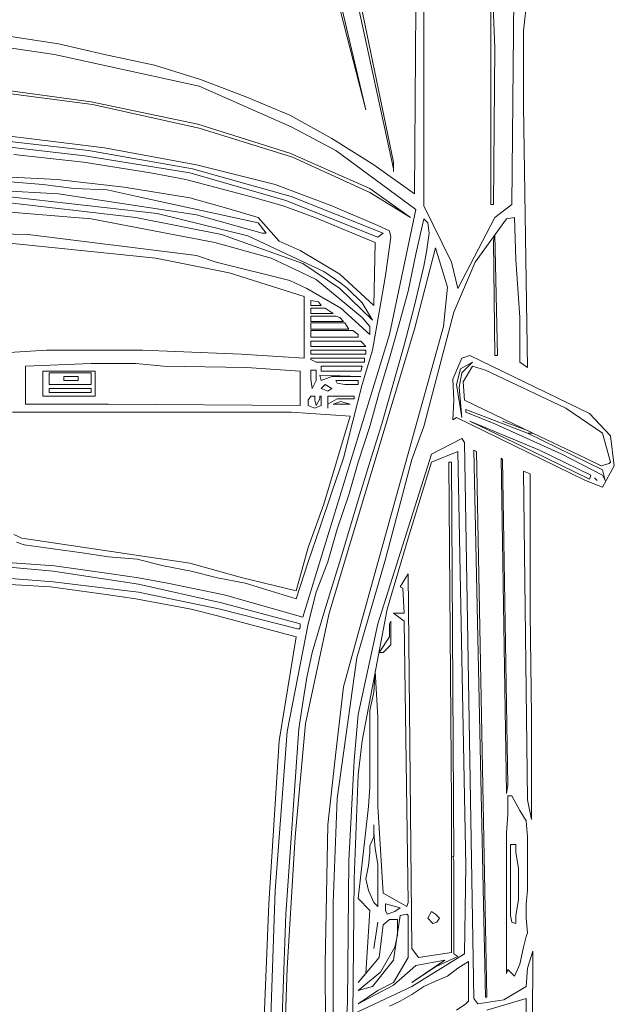
# Model space of a CAD drawing. Units: inches. Extents: x -9 to 646, y -802 to 47.
# Tile 8 of 17: x 465 to 490, y -602 to -561. Entities that reach past the tile are written whole.
import ezdxf

# ---------------------------------------------------------------- set-up
doc = ezdxf.new("R2010")
doc.units = ezdxf.units.IN
doc.header["$MEASUREMENT"] = 0
doc.layers.add('A-SITE-VEHI', color=8, linetype='Continuous', lineweight=9)

msp = doc.modelspace()

# ---------------------------------------------------------------- linework, layer by layer
at = {"layer": 'A-SITE-VEHI'}
for p, q in [((474.722, -545.354), (479.383, -565.082)), ((484.206, -549.797), (484.694, -562.536)), ((480.522, -567.521), (476.836, -550.556)), ((481.767, -550.827), (481.767, -569.039)), ((477.54, -552.941), (480.522, -567.25)), ((485.398, -568.984), (485.507, -558.523)), ((479.383, -565.082), (477.811, -558.958)), ((485.886, -561.83), (486.048, -560.313)), ((481.388, -568.551), (481.443, -560.855)), ((484.532, -568.984), (484.532, -560.964)), ((485.886, -564.92), (485.886, -561.83)), ((466.537, -562.806), (462.418, -562.209)), ((464.639, -562.047), (466.699, -562.371)), ((466.699, -562.371), (468.596, -562.806)), ((484.694, -562.536), (484.641, -568.984)), ((472.499, -564.108), (466.537, -562.806)), ((468.596, -562.806), (470.656, -563.239)), ((470.656, -563.239), (472.553, -563.835)), ((472.553, -563.835), (474.396, -564.541)), ((463.069, -564.214), (468.109, -564.865)), ((468.054, -564.756), (463.231, -564.108)), ((476.294, -565.786), (472.499, -564.108)), ((474.396, -564.541), (476.239, -565.3)), ((472.444, -565.678), (468.054, -564.756)), ((468.109, -564.865), (472.499, -565.842)), ((486.048, -575.705), (485.886, -564.92)), ((476.239, -565.3), (477.973, -566.275)), ((476.239, -566.87), (472.444, -565.678)), ((472.499, -565.842), (476.347, -567.034)), ((478.137, -566.763), (476.294, -565.786)), ((467.945, -566.763), (463.611, -566.275)), ((468.596, -566.655), (464.694, -566.166)), ((477.973, -566.275), (479.707, -567.358)), ((463.502, -566.492), (467.783, -566.979)), ((472.39, -567.358), (468.596, -566.655)), ((467.73, -567.25), (464.856, -566.925)), ((467.783, -566.979), (472.12, -567.685)), ((472.228, -567.521), (467.945, -566.763)), ((479.545, -568.335), (476.239, -566.87)), ((476.347, -567.034), (479.545, -568.497)), ((481.443, -569.201), (478.137, -566.763)), ((458.026, -567.521), (466.646, -567.956)), ((470.494, -567.685), (467.73, -567.25)), ((476.294, -568.66), (472.228, -567.521)), ((475.643, -568.171), (472.39, -567.358)), ((479.707, -567.358), (481.388, -568.551)), ((480.522, -567.25), (480.522, -567.629)), ((471.957, -567.956), (470.494, -567.685)), ((472.12, -567.685), (476.076, -568.822)), ((458.948, -568.118), (466.699, -568.551)), ((466.049, -568.171), (463.447, -567.956)), ((467.35, -568.335), (466.049, -568.171)), ((466.646, -567.956), (469.411, -568.28)), ((468.705, -568.389), (467.35, -568.335)), ((469.411, -568.28), (472.12, -568.713)), ((474.613, -568.66), (471.957, -567.956)), ((477.973, -569.039), (475.643, -568.171)), ((481.226, -569.528), (479.545, -568.335)), ((470.765, -569.364), (463.664, -568.551)), ((466.699, -568.551), (472.39, -569.419)), ((469.952, -568.66), (468.705, -568.389)), ((474.937, -569.743), (469.952, -568.66)), ((472.12, -568.713), (473.692, -569.148)), ((475.968, -569.039), (474.613, -568.66)), ((480.087, -570.176), (476.294, -568.66)), ((479.545, -568.497), (481.226, -569.528)), ((463.826, -568.822), (469.897, -569.528)), ((477.269, -569.528), (475.968, -569.039)), ((476.076, -568.822), (479.871, -570.34)), ((479.871, -569.852), (477.973, -569.039)), ((481.767, -569.039), (482.906, -571.369)), ((484.641, -568.984), (484.532, -568.984)), ((484.694, -569.528), (485.398, -568.984)), ((468.054, -569.581), (462.798, -569.148)), ((469.897, -569.528), (473.421, -570.232)), ((474.504, -570.285), (470.765, -569.364)), ((472.39, -569.419), (475.102, -570.176)), ((473.692, -569.148), (474.937, -569.528)), ((474.937, -569.528), (475.806, -570.503)), ((479.762, -570.556), (477.269, -569.528)), ((480.357, -574.351), (481.443, -569.201)), ((483.177, -572.454), (484.694, -569.528)), ((485.182, -569.581), (485.507, -569.528)), ((485.507, -569.528), (485.562, -571.262)), ((473.15, -570.556), (468.054, -569.581)), ((475.264, -570.176), (474.937, -569.743)), ((480.357, -570.07), (479.871, -569.852)), ((481.767, -569.581), (481.443, -571.044)), ((481.93, -569.743), (481.767, -569.581)), ((481.985, -570.176), (481.93, -569.743)), ((483.881, -571.369), (485.182, -569.581)), ((463.069, -570.176), (465.454, -570.232)), ((465.454, -570.232), (472.39, -571.098)), ((473.421, -570.232), (476.78, -571.424)), ((477.648, -571.748), (474.504, -570.285)), ((475.102, -570.176), (475.264, -570.176)), ((479.871, -570.34), (480.087, -570.176)), ((480.195, -571.913), (480.413, -570.34)), ((480.413, -570.34), (480.357, -570.07)), ((481.876, -570.936), (481.985, -570.176)), ((484.694, -570.232), (484.641, -570.503)), ((484.803, -575.219), (484.694, -570.232)), ((470.71, -571.206), (464.423, -570.556)), ((475.479, -571.206), (473.15, -570.556)), ((475.806, -570.503), (476.672, -570.882)), ((479.707, -573.158), (479.762, -570.556)), ((484.641, -570.503), (484.694, -575.219)), ((472.39, -571.098), (473.203, -571.369)), ((476.672, -570.882), (478.299, -571.857)), ((481.443, -571.044), (481.117, -572.561)), ((481.388, -574.133), (482.256, -570.773)), ((481.767, -571.533), (481.876, -570.936)), ((482.256, -570.773), (482.742, -572.399)), ((473.745, -571.804), (470.71, -571.206)), ((473.203, -571.369), (476.239, -572.128)), ((476.401, -571.642), (475.479, -571.206)), ((476.78, -571.424), (478.299, -572.454)), ((481.388, -573.158), (481.767, -571.533)), ((482.906, -571.369), (483.177, -572.454)), ((483.013, -573.429), (483.881, -571.369)), ((485.562, -571.262), (485.724, -573.647)), ((476.836, -572.779), (473.745, -571.804)), ((477.322, -572.075), (476.401, -571.642)), ((478.352, -572.237), (477.648, -571.748)), ((478.299, -571.857), (479.707, -573.158)), ((479.924, -573.429), (480.195, -571.913)), ((476.239, -572.128), (476.945, -572.454)), ((479.221, -573.647), (477.322, -572.075)), ((478.623, -572.454), (478.352, -572.237)), ((476.836, -575.325), (476.836, -572.779)), ((476.945, -572.454), (478.352, -573.267)), ((478.299, -572.454), (479.654, -573.755)), ((479.221, -573.049), (478.623, -572.454)), ((481.117, -572.561), (480.737, -573.971)), ((482.742, -572.399), (482.58, -574.026)), ((477.431, -572.996), (477.107, -572.941)), ((477.107, -572.941), (477.107, -573.158)), ((477.107, -573.158), (477.54, -573.158)), ((477.54, -573.158), (477.431, -572.996)), ((479.654, -573.755), (479.221, -573.049)), ((480.955, -574.784), (481.388, -573.158)), ((477.702, -573.267), (477.107, -573.267)), ((477.107, -573.267), (477.107, -573.482)), ((477.107, -573.482), (478.028, -573.482)), ((478.137, -573.591), (477.107, -573.591)), ((477.107, -573.591), (477.107, -573.809)), ((478.028, -573.482), (477.702, -573.267)), ((478.299, -573.647), (478.137, -573.591)), ((478.352, -573.267), (479.545, -574.351)), ((479.654, -575.001), (479.924, -573.429)), ((481.767, -578.145), (483.013, -573.429)), ((477.107, -573.809), (478.461, -573.809)), ((478.514, -573.862), (477.107, -573.862)), ((477.107, -573.862), (477.107, -574.133)), ((478.461, -573.809), (478.299, -573.647)), ((478.679, -574.133), (478.514, -573.862)), ((479.545, -574.026), (479.221, -573.647)), ((480.737, -573.971), (480.357, -575.325)), ((485.724, -573.647), (485.724, -575.49)), ((476.78, -586.004), (480.357, -574.351)), ((477.107, -574.133), (478.679, -574.133)), ((478.841, -574.189), (477.107, -574.189)), ((477.107, -574.189), (477.107, -574.459)), ((477.864, -585.841), (481.388, -574.133)), ((479.058, -574.351), (478.841, -574.189)), ((479.058, -574.459), (479.058, -574.351)), ((482.58, -574.026), (479.165, -586.274)), ((479.545, -574.351), (479.545, -574.026)), ((477.107, -574.459), (479.058, -574.459)), ((479.165, -574.622), (477.107, -574.622)), ((477.107, -574.622), (477.107, -574.839)), ((479.221, -574.675), (479.165, -574.622)), ((479.383, -574.839), (479.221, -574.675)), ((480.033, -578.037), (480.955, -574.784)), ((463.502, -575.163), (466.211, -575.001)), ((466.211, -575.001), (470.168, -575.001)), ((470.168, -575.001), (471.524, -575.055)), ((471.524, -575.055), (474.233, -575.163)), ((474.233, -575.163), (476.836, -575.325)), ((477.107, -574.839), (479.383, -574.839)), ((479.383, -575.001), (477.107, -575.001)), ((477.107, -575.001), (477.107, -575.163)), ((477.107, -575.163), (479.383, -575.163)), ((479.221, -576.411), (479.654, -575.001)), ((479.383, -575.163), (479.383, -575.001)), ((483.664, -575.219), (483.339, -575.325)), ((488.597, -577.604), (483.664, -575.219)), ((484.694, -575.219), (484.803, -575.219)), ((468.054, -575.543), (465.345, -575.652)), ((469.897, -575.543), (468.054, -575.543)), ((471.036, -575.652), (469.897, -575.543)), ((479.329, -575.325), (477.107, -575.325)), ((477.107, -575.325), (477.107, -575.381)), ((477.107, -575.381), (477.322, -575.49)), ((477.322, -575.49), (479.329, -575.49)), ((479.329, -575.49), (479.329, -575.325)), ((480.357, -575.325), (479.924, -576.735)), ((483.339, -575.325), (482.96, -576.194)), ((483.772, -575.49), (483.284, -575.761)), ((483.339, -575.923), (483.772, -575.49)), ((485.724, -575.49), (486.048, -575.705)), ((465.345, -575.652), (465.345, -577.224)), ((468.218, -575.867), (466.049, -575.867)), ((466.049, -575.867), (466.049, -576.897)), ((468.054, -575.923), (466.32, -575.923)), ((466.32, -575.923), (466.32, -576.411)), ((468.054, -576.411), (468.054, -575.923)), ((468.218, -576.897), (468.218, -575.867)), ((474.451, -575.705), (471.036, -575.652)), ((476.672, -575.867), (474.451, -575.705)), ((476.672, -577.277), (476.672, -575.867)), ((477.322, -575.814), (477.107, -575.814)), ((477.107, -575.814), (477.107, -576.194)), ((477.322, -576.247), (477.322, -575.814)), ((479.165, -576.085), (477.486, -576.031)), ((477.486, -576.031), (477.54, -576.247)), ((479.221, -575.652), (477.54, -575.652)), ((477.54, -575.652), (477.54, -575.867)), ((477.54, -575.867), (479.165, -575.867)), ((479.165, -575.867), (479.221, -575.652)), ((483.284, -575.761), (483.122, -576.411)), ((483.231, -576.518), (483.339, -575.923)), ((483.772, -575.652), (483.393, -576.302)), ((484.314, -575.814), (483.772, -575.652)), ((487.621, -577.386), (484.314, -575.814)), ((466.32, -576.411), (468.054, -576.411)), ((467.512, -576.085), (466.917, -576.085)), ((466.917, -576.085), (466.917, -576.247)), ((466.917, -576.247), (467.512, -576.247)), ((467.512, -576.247), (467.512, -576.085)), ((477.107, -576.194), (477.16, -576.573)), ((477.16, -576.573), (477.322, -576.247)), ((477.54, -576.247), (477.973, -576.085)), ((477.702, -576.411), (477.54, -576.573)), ((477.973, -576.573), (477.702, -576.411)), ((477.973, -576.085), (479.165, -576.085)), ((479.058, -576.247), (478.137, -576.247)), ((478.137, -576.247), (478.19, -576.356)), ((478.19, -576.356), (478.514, -576.411)), ((478.514, -576.411), (479.058, -576.411)), ((478.841, -577.928), (479.221, -576.411)), ((479.058, -576.411), (479.058, -576.247)), ((482.96, -576.194), (483.013, -577.062)), ((483.122, -576.411), (483.339, -577.766)), ((483.393, -576.302), (483.448, -577.062)), ((468.054, -576.573), (466.32, -576.573)), ((466.32, -576.573), (466.32, -576.735)), ((466.32, -576.735), (468.054, -576.735)), ((468.054, -576.735), (468.054, -576.573)), ((477.54, -576.573), (477.811, -576.682)), ((477.811, -576.682), (477.973, -576.573)), ((479.924, -576.735), (479.545, -578.145)), ((483.339, -577.766), (483.231, -576.518)), ((465.345, -577.224), (468.76, -577.224)), ((466.049, -576.897), (468.218, -576.897)), ((468.76, -577.224), (476.672, -577.277)), ((477.107, -576.897), (476.998, -577.062)), ((476.998, -577.062), (476.998, -577.277)), ((477.269, -576.897), (477.107, -576.897)), ((477.269, -577.062), (477.269, -576.897)), ((477.322, -577.277), (477.269, -577.062)), ((477.486, -577.006), (477.322, -577.277)), ((477.54, -576.897), (477.486, -576.897)), ((477.486, -576.897), (477.486, -577.006)), ((477.54, -577.277), (477.54, -576.897)), ((478.894, -576.897), (477.811, -576.897)), ((477.811, -576.897), (477.811, -577.386)), ((477.811, -577.224), (478.19, -577.006)), ((478.352, -577.115), (478.028, -577.224)), ((478.028, -577.224), (478.732, -577.224)), ((478.19, -577.006), (478.894, -577.006)), ((478.732, -577.224), (478.352, -577.115)), ((478.894, -577.006), (478.894, -576.897)), ((483.013, -577.062), (482.96, -577.874)), ((483.448, -577.062), (486.266, -578.416)), ((476.294, -577.548), (464.803, -577.548)), ((478.732, -577.71), (476.294, -577.548)), ((476.998, -577.277), (477.269, -577.386)), ((477.269, -577.386), (477.54, -577.277)), ((486.048, -578.416), (483.502, -577.439)), ((483.502, -577.439), (483.502, -577.548)), ((483.502, -577.548), (484.694, -578.037)), ((489.139, -578.416), (487.621, -577.386)), ((489.464, -578.525), (488.597, -577.604)), ((477.648, -581.343), (478.732, -577.71)), ((478.461, -579.447), (478.841, -577.928)), ((479.545, -579.609), (480.033, -578.037)), ((482.96, -577.874), (483.122, -577.766)), ((483.122, -577.766), (488.433, -580.368)), ((483.664, -577.928), (486.266, -579.176)), ((486.537, -579.12), (483.664, -577.928)), ((484.694, -578.037), (487.458, -579.282)), ((485.02, -577.928), (486.048, -578.307)), ((479.545, -578.145), (479.058, -579.609)), ((481.279, -579.5), (481.767, -578.145)), ((489.139, -579.933), (486.048, -578.416)), ((486.048, -578.416), (486.266, -578.416)), ((486.266, -578.416), (488.433, -579.447)), ((489.464, -579.609), (489.139, -578.416)), ((483.339, -578.632), (482.092, -579.282)), ((483.448, -578.796), (483.339, -578.632)), ((483.828, -601.722), (483.448, -578.796)), ((489.626, -579.771), (489.464, -578.525)), ((482.092, -579.282), (479.871, -586.274)), ((483.177, -579.176), (482.092, -579.609)), ((483.502, -596.249), (483.177, -579.176)), ((483.935, -579.176), (483.828, -579.12)), ((483.828, -579.12), (484.314, -601.669)), ((484.37, -601.669), (483.935, -579.176)), ((486.266, -579.176), (488.597, -580.313)), ((488.651, -580.15), (486.537, -579.12)), ((487.458, -579.282), (489.139, -580.15)), ((477.973, -580.854), (478.461, -579.447)), ((479.058, -579.609), (478.679, -580.963)), ((479.058, -581.181), (479.545, -579.609)), ((480.195, -583.619), (481.279, -579.5)), ((482.092, -579.609), (481.117, -582.753)), ((482.906, -579.609), (482.798, -579.609)), ((482.798, -579.609), (482.906, -593.7)), ((483.013, -595.869), (482.906, -579.609)), ((485.02, -579.5), (484.965, -579.447)), ((484.965, -579.447), (485.182, -593.267)), ((485.236, -592.942), (485.02, -579.5)), ((488.433, -579.447), (489.084, -579.771)), ((489.084, -579.771), (489.41, -579.662)), ((489.41, -579.662), (489.464, -579.609)), ((486.157, -580.095), (485.886, -579.988)), ((485.886, -579.988), (486.048, -593.538)), ((486.157, -585.841), (486.157, -580.095)), ((489.139, -580.639), (489.626, -579.771)), ((489.248, -580.368), (489.139, -579.933)), ((488.433, -580.368), (489.139, -580.639)), ((488.597, -580.313), (488.651, -580.15)), ((488.813, -580.259), (488.922, -580.368)), ((489.139, -580.15), (489.248, -580.368)), ((477.486, -582.318), (477.973, -580.854)), ((478.679, -580.963), (478.19, -582.373)), ((478.352, -583.565), (479.058, -581.181)), ((476.998, -583.13), (477.648, -581.343)), ((476.998, -583.728), (477.486, -582.318)), ((478.19, -582.373), (477.811, -583.728)), ((464.856, -582.589), (465.183, -582.753)), ((464.965, -582.915), (465.29, -583.024)), ((465.183, -582.753), (472.12, -583.781)), ((481.117, -582.753), (480.251, -585.679)), ((465.29, -583.024), (467.674, -583.348)), ((467.674, -583.348), (468.76, -583.51)), ((476.509, -584.92), (476.998, -583.13)), ((462.905, -583.619), (466.537, -583.89)), ((468.76, -583.51), (469.952, -583.619)), ((469.952, -583.619), (471.036, -583.89)), ((476.509, -585.244), (476.998, -583.728)), ((477.811, -583.728), (477.322, -584.973)), ((477.648, -585.841), (478.352, -583.565)), ((479.003, -587.684), (480.195, -583.619)), ((466.482, -584.107), (462.905, -583.781)), ((470.006, -584.649), (466.482, -584.107)), ((466.537, -583.89), (468.867, -584.216)), ((471.036, -583.89), (472.173, -584.107)), ((472.12, -583.781), (474.287, -584.378)), ((472.173, -584.107), (473.259, -584.378)), ((466.375, -584.758), (462.798, -584.54)), ((462.905, -584.269), (466.482, -584.54)), ((466.482, -584.54), (470.006, -584.973)), ((468.867, -584.216), (470.006, -584.378)), ((470.006, -584.378), (471.198, -584.596)), ((473.259, -584.378), (474.396, -584.596)), ((474.287, -584.378), (476.509, -584.92)), ((481.117, -584.216), (480.793, -584.758)), ((481.279, -599.662), (481.117, -584.216)), ((468.76, -585.082), (466.375, -584.758)), ((473.421, -585.408), (470.006, -584.649)), ((470.006, -584.973), (473.365, -585.679)), ((471.198, -584.596), (473.53, -585.082)), ((474.396, -584.596), (475.426, -584.92)), ((475.426, -584.92), (476.509, -585.244)), ((477.322, -584.973), (476.998, -586.274)), ((480.793, -584.758), (480.899, -584.811)), ((480.899, -584.811), (480.955, -585.841)), ((469.897, -585.244), (468.76, -585.082)), ((472.173, -585.679), (469.897, -585.244)), ((473.53, -585.082), (476.78, -586.004)), ((473.259, -585.95), (472.173, -585.679)), ((473.365, -585.679), (476.618, -586.492)), ((476.672, -586.274), (473.421, -585.408)), ((480.251, -585.679), (479.221, -591.099)), ((476.509, -586.816), (473.259, -585.95)), ((476.889, -590.393), (477.864, -585.841)), ((477.16, -587.467), (477.648, -585.841)), ((480.413, -586.166), (480.357, -586.274)), ((480.413, -587.143), (480.413, -586.166)), ((480.955, -585.841), (480.522, -585.841)), ((480.522, -585.841), (480.955, -586.166)), ((480.955, -586.166), (481.117, -597.765)), ((486.213, -590.069), (486.157, -585.841)), ((476.998, -586.274), (476.13, -590.72)), ((476.618, -586.492), (476.672, -586.437)), ((476.672, -586.437), (476.672, -586.274)), ((479.165, -586.274), (478.461, -588.877)), ((479.871, -586.274), (479.058, -590.016)), ((480.357, -586.274), (480.357, -586.816)), ((475.806, -591.099), (476.509, -586.816)), ((480.357, -586.816), (479.924, -587.467)), ((480.087, -587.467), (480.413, -587.143)), ((476.945, -588.497), (477.16, -587.467)), ((478.19, -593.484), (479.003, -587.684)), ((479.924, -587.467), (480.087, -587.467)), ((479.762, -588.226), (479.707, -589.094)), ((479.871, -590.122), (479.762, -588.226)), ((476.78, -589.527), (476.945, -588.497)), ((478.461, -588.877), (478.137, -591.586)), ((479.707, -589.094), (479.545, -589.852)), ((476.618, -590.611), (476.78, -589.527)), ((479.058, -590.016), (478.894, -591.912)), ((479.545, -589.852), (479.545, -592.996)), ((479.871, -593.808), (479.871, -590.122)), ((486.213, -594.35), (486.213, -590.069)), ((476.076, -598.254), (476.618, -590.611)), ((476.456, -595.056), (476.889, -590.393)), ((476.13, -590.72), (475.643, -597.277)), ((475.372, -597.821), (475.806, -591.099)), ((479.221, -591.099), (479.058, -592.507)), ((478.137, -591.586), (477.811, -594.568)), ((478.894, -591.912), (478.679, -596.031)), ((479.058, -592.507), (478.894, -596.79)), ((479.545, -592.996), (479.491, -593.808)), ((485.182, -593.267), (485.236, -592.942)), ((478.028, -597.765), (478.19, -593.484)), ((485.398, -593.375), (485.236, -593.375)), ((485.236, -593.375), (485.236, -594.135)), ((485.724, -593.971), (485.398, -593.375)), ((479.491, -593.808), (479.058, -597.603)), ((480.087, -597.386), (479.871, -593.808)), ((482.906, -593.7), (482.906, -599.826)), ((486.048, -593.538), (486.213, -594.35)), ((485.236, -594.135), (485.182, -594.892)), ((485.995, -594.406), (485.724, -593.971)), ((477.811, -594.568), (477.702, -600.312)), ((479.707, -594.568), (479.707, -595.056)), ((486.048, -595.056), (485.995, -594.406)), ((476.13, -600.476), (476.456, -595.056)), ((479.707, -595.056), (479.545, -595.436)), ((479.762, -595.543), (479.707, -594.892)), ((485.182, -594.892), (485.182, -600.692)), ((486.048, -597.277), (486.048, -595.056)), ((479.545, -595.436), (479.545, -595.707)), ((485.562, -595.38), (485.345, -595.38)), ((485.345, -595.38), (485.345, -598.307)), ((485.562, -595.707), (485.562, -595.38)), ((479.545, -595.707), (479.491, -596.249)), ((479.871, -596.193), (479.762, -595.543)), ((483.013, -596.031), (482.96, -595.869)), ((482.96, -595.869), (483.013, -595.869)), ((485.671, -596.355), (485.562, -595.707)), ((478.679, -596.031), (478.623, -601.884)), ((479.491, -596.249), (479.383, -596.79)), ((479.871, -597.927), (479.871, -596.193)), ((483.013, -599.879), (483.013, -596.031)), ((483.448, -599.879), (483.502, -596.249)), ((485.671, -597.656), (485.671, -596.355)), ((478.894, -596.79), (478.841, -602.373)), ((479.383, -596.79), (479.491, -597.277)), ((475.643, -597.277), (474.451, -630.612)), ((479.491, -597.277), (479.707, -597.765)), ((481.064, -597.927), (480.087, -597.386)), ((485.995, -597.821), (486.048, -597.277)), ((475.102, -604.487), (475.372, -597.821)), ((478.028, -603.727), (478.028, -597.765)), ((479.058, -597.603), (479.545, -598.092)), ((479.707, -597.765), (479.871, -597.927)), ((480.793, -597.983), (480.195, -597.821)), ((480.195, -597.821), (480.195, -598.092)), ((481.117, -597.765), (481.064, -597.927)), ((485.562, -598.307), (485.671, -597.656)), ((485.995, -598.416), (485.995, -597.821)), ((474.884, -630.612), (476.076, -598.254)), ((479.545, -598.092), (479.383, -600.692)), ((480.195, -598.092), (480.251, -598.254)), ((480.251, -598.254), (480.575, -598.145)), ((480.522, -600.15), (480.793, -598.307)), ((480.575, -598.145), (480.793, -597.983)), ((480.793, -598.307), (481.064, -598.254)), ((481.064, -598.254), (481.117, -598.307)), ((481.117, -598.307), (481.117, -600.041)), ((482.092, -598.145), (481.93, -598.416)), ((482.256, -598.254), (482.092, -598.145)), ((482.418, -598.416), (482.256, -598.254)), ((485.345, -598.307), (485.398, -598.578)), ((485.562, -598.633), (485.562, -598.307)), ((479.707, -599.662), (479.871, -598.578)), ((479.924, -600.041), (480.087, -598.687)), ((480.087, -598.687), (480.357, -598.469)), ((480.357, -598.469), (480.684, -598.469)), ((480.684, -598.469), (480.684, -599.12)), ((481.93, -598.416), (482.147, -598.633)), ((482.147, -598.633), (482.309, -598.578)), ((482.309, -598.578), (482.418, -598.416)), ((485.398, -598.578), (485.562, -598.633)), ((486.048, -599.013), (485.995, -598.416)), ((480.684, -599.12), (480.575, -599.608)), ((485.886, -599.608), (485.995, -599.175)), ((485.995, -599.175), (486.048, -599.013)), ((480.575, -599.608), (479.978, -600.638)), ((481.55, -600.041), (481.279, -599.662)), ((481.279, -601.234), (483.448, -599.879)), ((482.906, -599.826), (481.55, -600.041)), ((482.256, -600.421), (483.177, -599.988)), ((483.177, -599.988), (483.013, -599.879)), ((485.724, -600.312), (485.886, -599.608)), ((486.266, -599.77), (486.048, -600.476)), ((486.213, -613.808), (486.266, -599.77)), ((477.702, -600.312), (477.811, -615.869)), ((479.058, -601.071), (479.924, -600.041)), ((479.654, -601.234), (480.522, -600.15)), ((481.117, -600.041), (480.522, -601.071)), ((480.522, -601.18), (481.443, -600.368)), ((482.636, -600.15), (481.279, -601.071)), ((481.443, -600.368), (482.636, -600.15)), ((483.177, -600.476), (483.61, -600.205)), ((483.61, -600.205), (483.61, -601.831)), ((485.507, -600.801), (485.724, -600.312)), ((475.208, -629.635), (476.13, -600.476)), ((479.978, -600.638), (479.058, -601.398)), ((479.383, -600.692), (479.058, -601.071)), ((481.279, -601.071), (482.256, -600.421)), ((482.256, -601.018), (482.742, -600.801)), ((482.742, -600.801), (483.177, -600.476)), ((485.182, -600.692), (485.236, -600.53)), ((485.236, -600.53), (485.507, -600.801)), ((486.048, -600.476), (485.995, -601.234)), ((479.058, -601.94), (480.522, -601.18)), ((480.522, -601.071), (479.871, -601.398)), ((481.767, -601.234), (482.256, -601.018)), ((478.841, -602.373), (481.279, -601.234)), ((479.058, -601.398), (479.654, -601.234)), ((479.871, -601.398), (479.058, -601.94)), ((480.793, -601.831), (481.279, -601.56)), ((481.279, -601.56), (481.767, -601.234)), ((485.995, -601.234), (485.074, -601.775)), ((478.623, -601.884), (478.514, -603.727)), ((480.357, -602.048), (480.793, -601.831)), ((483.502, -601.94), (483.122, -602.211)), ((483.61, -601.831), (483.502, -601.94)), ((483.99, -601.94), (483.828, -601.722)), ((485.074, -601.775), (483.99, -601.94)), ((484.314, -601.669), (484.37, -601.669)), ((484.37, -602.211), (485.995, -601.722)), ((485.995, -601.722), (485.833, -621.071))]:
    msp.add_line(p, q, dxfattribs=at)

doc.saveas('drawing.dxf')
